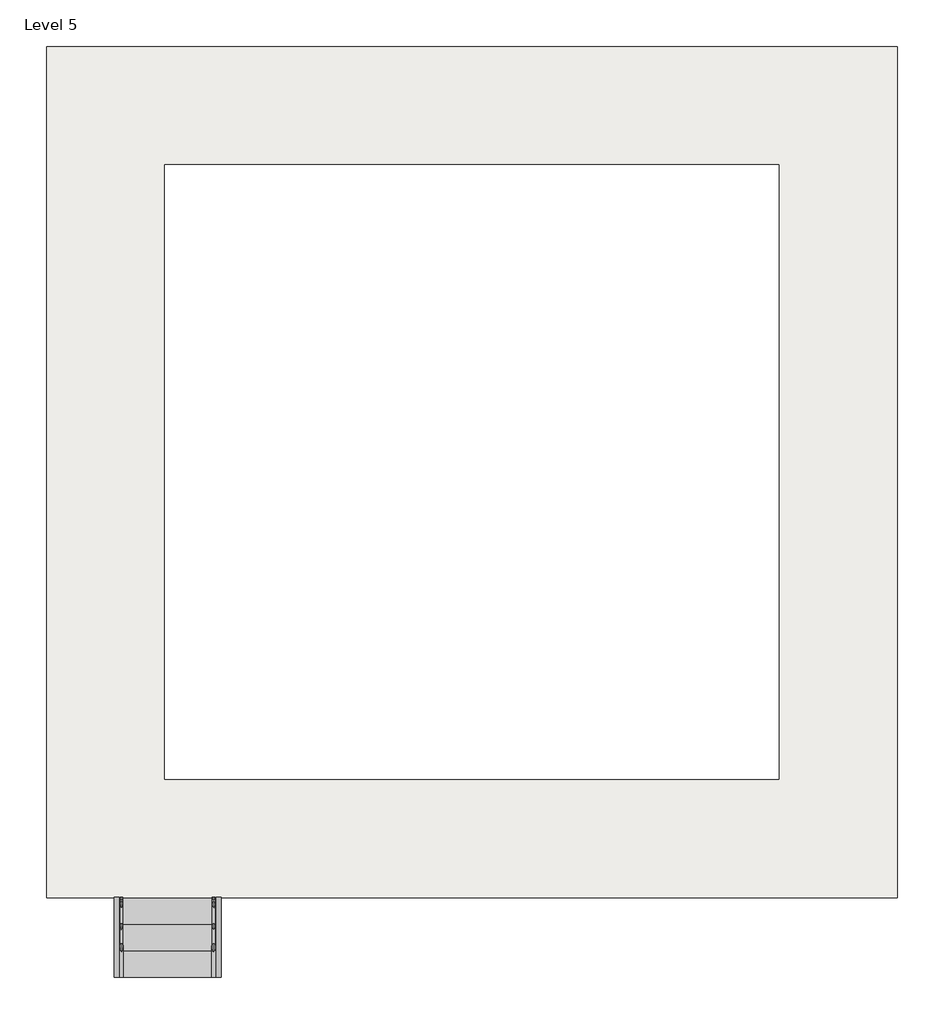
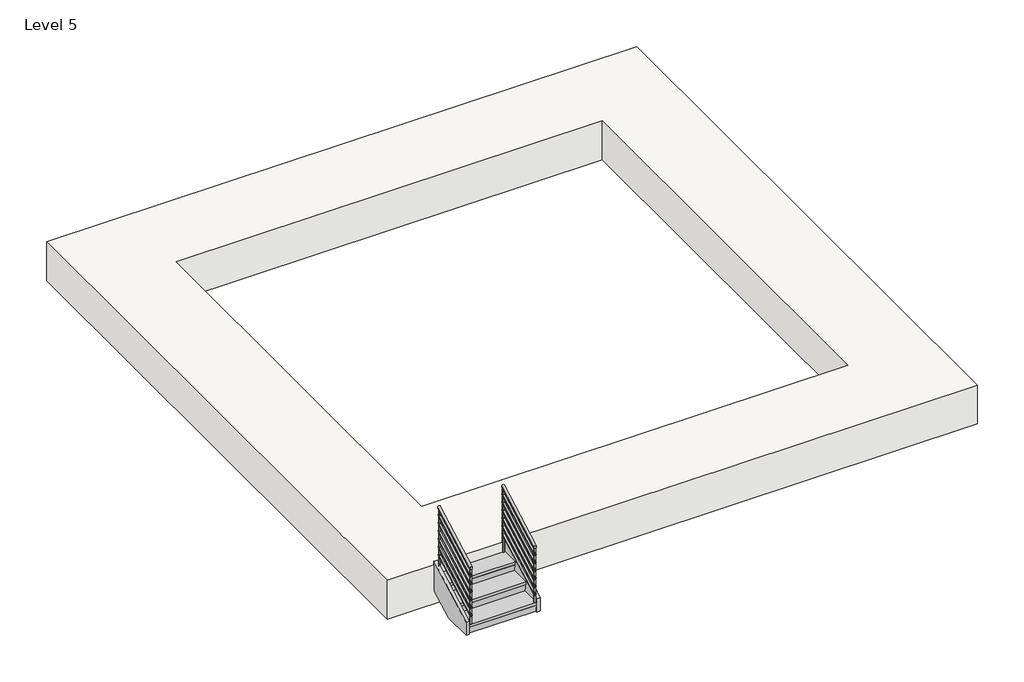
# One storey: 2 members, 2 railings, 1 slab, 1 stair flight.
"""IFC4 building model written with IfcOpenShell, lengths in millimetres."""

from ifc_helpers import new_model, si_unit, frame, origin, place, context, project, spatial, polyline, circle_curve, ellipse_curve, outline, extrude, transform, mapped, element, save
from ifc_brep_helpers import plane_surface, cylinder_surface, advanced_brep
from components import stair_flight_50mm_tread_25mm_nosing_13mm_riser_f84e0c27

model = new_model("IFC4")

# Units and contexts
model_context = context("Model", 3, world=origin())
ifc_project = project(units=[si_unit("LENGTHUNIT", "METRE", prefix="MILLI")], contexts=[model_context])

# Site, building, storey
site = spatial("IfcSite", under=ifc_project)
building = spatial("IfcBuilding", under=site)
storey = spatial("IfcBuildingStorey", under=building, Name="Level 5", Elevation=-609.6)

# Members
placement = place(None, origin())
element("IfcMember", 1, ObjectType="Stringer - 50mm Width", at=placement, inside=storey, context=model_context, shape_type="SweptSolid", body=[
    extrude(outline(polyline([(-5656.14356, -609.6), (-5656.14356, -401.4833471), (-4831.14356, 55.7166529), (-4831.14356, -401.6003029), (-5206.4710976, -609.6), (-5656.14356, -609.6)])), frame((-15823.6523905, 0.0, 0.0), z_axis=(1.0, 0.0, 0.0), x_axis=(0.0, 1.0, 0.0)), (0.0, 0.0, 1.0), 50.0),
])
element("IfcMember", 2, ObjectType="Stringer - 50mm Width", at=placement, inside=storey, context=model_context, shape_type="SweptSolid", body=[
    extrude(outline(polyline([(-5656.14356, -609.6), (-5656.14356, -401.4833471), (-4831.14356, 55.7166529), (-4831.14356, -401.6003029), (-5206.4710976, -609.6), (-5656.14356, -609.6)])), frame((-14773.6266093, 0.0, 0.0), z_axis=(1.0, 0.0, 0.0), x_axis=(0.0, 1.0, 0.0)), (0.0, 0.0, 1.0), 50.0),
])

# Railings
element("IfcRailing", 3, ObjectType="900mm Pipe", at=placement, inside=storey, context=model_context, shape_type="AdvancedBrep", body=[
    advanced_brep(
    [(-14779.0266093, -5656.14356, 419.9341522), (-14819.0266093, -5656.14356, 419.9341522), (-14779.0266093, -4831.14356, 877.1341522), (-14819.0266093, -4831.14356, 877.1341522)],
    [
        (0, 1, ellipse_curve(frame((-14799.0266093, -5656.14356, 419.9341522), z_axis=(0.0, -1.0, 0.0), x_axis=(0.0, 0.0, -0.9999999999999999)), 22.8658478, 20.0)),
        (1, 0, ellipse_curve(frame((-14799.0266093, -5656.14356, 419.9341522), z_axis=(0.0, -1.0, 0.0), x_axis=(0.0, 0.0, -0.9999999999999999)), 22.8658478, 20.0)),
        (2, 3, ellipse_curve(frame((-14799.0266093, -4831.14356, 877.1341522), z_axis=(0.0, 1.0, 0.0), x_axis=(0.0, 0.0, -0.9999999999999999)), 22.8658478, 20.0)),
        (3, 2, ellipse_curve(frame((-14799.0266093, -4831.14356, 877.1341522), z_axis=(0.0, 1.0, 0.0), x_axis=(0.0, 0.0, -0.9999999999999999)), 22.8658478, 20.0)),
        (0, 2),
        (3, 1),
    ],
    [
        plane_surface(frame((-14799.0266093, -5656.14356, 442.8), z_axis=(0.0, -1.0, 0.0), x_axis=(0.0, 0.0, 1.0))),
        plane_surface(frame((-14799.0266093, -4831.14356, 900.0), z_axis=(0.0, 1.0, 0.0), x_axis=(0.0, 0.0, 1.0))),
        cylinder_surface(frame((-14799.0266093, -5646.4490703, 425.3066622), z_axis=(0.0, -0.8746668912460589, -0.48472448809396357), x_axis=(-1.0, 0.0, 0.0)), 20.0),
    ],
    [
        (0, [[1, 2]]),
        (1, [[3, 4]]),
        (2, [[-1, 5, -4, 6]]),
        (2, [[-2, -6, -3, -5]]),
    ],
),
    advanced_brep(
    [(-14814.0266093, -5656.14356, 300.6506142), (-14784.0266093, -5656.14356, 300.6506142), (-14814.0266093, -4831.14356, 757.8506142), (-14784.0266093, -4831.14356, 757.8506142)],
    [
        (0, 1, ellipse_curve(frame((-14799.0266093, -5656.14356, 300.6506142), z_axis=(0.0, -1.0, 0.0), x_axis=(0.0, 0.0, -0.9999999999999999)), 17.1493858, 15.0)),
        (1, 0, ellipse_curve(frame((-14799.0266093, -5656.14356, 300.6506142), z_axis=(0.0, -1.0, 0.0), x_axis=(0.0, 0.0, -0.9999999999999999)), 17.1493858, 15.0)),
        (2, 3, ellipse_curve(frame((-14799.0266093, -4831.14356, 757.8506142), z_axis=(0.0, 1.0, 0.0), x_axis=(0.0, 0.0, -0.9999999999999999)), 17.1493858, 15.0)),
        (3, 2, ellipse_curve(frame((-14799.0266093, -4831.14356, 757.8506142), z_axis=(0.0, 1.0, 0.0), x_axis=(0.0, 0.0, -0.9999999999999999)), 17.1493858, 15.0)),
        (0, 2),
        (3, 1),
    ],
    [
        plane_surface(frame((-14799.0266093, -5656.14356, 317.8), z_axis=(0.0, -1.0, 0.0), x_axis=(0.0, 0.0, 1.0))),
        plane_surface(frame((-14799.0266093, -4831.14356, 775.0), z_axis=(0.0, 1.0, 0.0), x_axis=(0.0, 0.0, 1.0))),
        cylinder_surface(frame((-14799.0266093, -5648.8726927, 304.6799966), z_axis=(0.0, -0.8746668912460589, -0.48472448809396357), x_axis=(1.0, 0.0, 0.0)), 15.0),
    ],
    [
        (0, [[1, 2]]),
        (1, [[3, 4]]),
        (2, [[-1, 5, -4, 6]]),
        (2, [[-2, -6, -3, -5]]),
    ],
),
    advanced_brep(
    [(-14814.0266093, -5656.14356, 175.6506142), (-14784.0266093, -5656.14356, 175.6506142), (-14814.0266093, -4831.14356, 632.8506142), (-14784.0266093, -4831.14356, 632.8506142)],
    [
        (0, 1, ellipse_curve(frame((-14799.0266093, -5656.14356, 175.6506142), z_axis=(0.0, -1.0, 0.0), x_axis=(0.0, 0.0, -0.9999999999999999)), 17.1493858, 15.0)),
        (1, 0, ellipse_curve(frame((-14799.0266093, -5656.14356, 175.6506142), z_axis=(0.0, -1.0, 0.0), x_axis=(0.0, 0.0, -0.9999999999999999)), 17.1493858, 15.0)),
        (2, 3, ellipse_curve(frame((-14799.0266093, -4831.14356, 632.8506142), z_axis=(0.0, 1.0, 0.0), x_axis=(0.0, 0.0, -0.9999999999999999)), 17.1493858, 15.0)),
        (3, 2, ellipse_curve(frame((-14799.0266093, -4831.14356, 632.8506142), z_axis=(0.0, 1.0, 0.0), x_axis=(0.0, 0.0, -0.9999999999999999)), 17.1493858, 15.0)),
        (0, 2),
        (3, 1),
    ],
    [
        plane_surface(frame((-14799.0266093, -5656.14356, 192.8), z_axis=(0.0, -1.0, 0.0), x_axis=(0.0, 0.0, 1.0))),
        plane_surface(frame((-14799.0266093, -4831.14356, 650.0), z_axis=(0.0, 1.0, 0.0), x_axis=(0.0, 0.0, 1.0))),
        cylinder_surface(frame((-14799.0266093, -5648.8726927, 179.6799966), z_axis=(0.0, -0.8746668912460589, -0.48472448809396357), x_axis=(1.0, 0.0, 0.0)), 15.0),
    ],
    [
        (0, [[1, 2]]),
        (1, [[3, 4]]),
        (2, [[-1, 5, -4, 6]]),
        (2, [[-2, -6, -3, -5]]),
    ],
),
    advanced_brep(
    [(-14814.0266093, -5656.14356, 50.6506142), (-14784.0266093, -5656.14356, 50.6506142), (-14814.0266093, -4831.14356, 507.8506142), (-14784.0266093, -4831.14356, 507.8506142)],
    [
        (0, 1, ellipse_curve(frame((-14799.0266093, -5656.14356, 50.6506142), z_axis=(0.0, -1.0, 0.0), x_axis=(0.0, 0.0, -0.9999999999999999)), 17.1493858, 15.0)),
        (1, 0, ellipse_curve(frame((-14799.0266093, -5656.14356, 50.6506142), z_axis=(0.0, -1.0, 0.0), x_axis=(0.0, 0.0, -0.9999999999999999)), 17.1493858, 15.0)),
        (2, 3, ellipse_curve(frame((-14799.0266093, -4831.14356, 507.8506142), z_axis=(0.0, 1.0, 0.0), x_axis=(0.0, 0.0, -0.9999999999999999)), 17.1493858, 15.0)),
        (3, 2, ellipse_curve(frame((-14799.0266093, -4831.14356, 507.8506142), z_axis=(0.0, 1.0, 0.0), x_axis=(0.0, 0.0, -0.9999999999999999)), 17.1493858, 15.0)),
        (0, 2),
        (3, 1),
    ],
    [
        plane_surface(frame((-14799.0266093, -5656.14356, 67.8), z_axis=(0.0, -1.0, 0.0), x_axis=(0.0, 0.0, 1.0))),
        plane_surface(frame((-14799.0266093, -4831.14356, 525.0), z_axis=(0.0, 1.0, 0.0), x_axis=(0.0, 0.0, 1.0))),
        cylinder_surface(frame((-14799.0266093, -5648.8726927, 54.6799966), z_axis=(0.0, -0.8746668912460589, -0.48472448809396357), x_axis=(1.0, 0.0, 0.0)), 15.0),
    ],
    [
        (0, [[1, 2]]),
        (1, [[3, 4]]),
        (2, [[-1, 5, -4, 6]]),
        (2, [[-2, -6, -3, -5]]),
    ],
),
    advanced_brep(
    [(-14814.0266093, -5656.14356, -74.3493858), (-14784.0266093, -5656.14356, -74.3493858), (-14814.0266093, -4831.14356, 382.8506142), (-14784.0266093, -4831.14356, 382.8506142)],
    [
        (0, 1, ellipse_curve(frame((-14799.0266093, -5656.14356, -74.3493858), z_axis=(0.0, -1.0, 0.0), x_axis=(0.0, 0.0, -0.9999999999999999)), 17.1493858, 15.0)),
        (1, 0, ellipse_curve(frame((-14799.0266093, -5656.14356, -74.3493858), z_axis=(0.0, -1.0, 0.0), x_axis=(0.0, 0.0, -0.9999999999999999)), 17.1493858, 15.0)),
        (2, 3, ellipse_curve(frame((-14799.0266093, -4831.14356, 382.8506142), z_axis=(0.0, 1.0, 0.0), x_axis=(0.0, 0.0, -0.9999999999999999)), 17.1493858, 15.0)),
        (3, 2, ellipse_curve(frame((-14799.0266093, -4831.14356, 382.8506142), z_axis=(0.0, 1.0, 0.0), x_axis=(0.0, 0.0, -0.9999999999999999)), 17.1493858, 15.0)),
        (0, 2),
        (3, 1),
    ],
    [
        plane_surface(frame((-14799.0266093, -5656.14356, -57.2), z_axis=(0.0, -1.0, 0.0), x_axis=(0.0, 0.0, 1.0))),
        plane_surface(frame((-14799.0266093, -4831.14356, 400.0), z_axis=(0.0, 1.0, 0.0), x_axis=(0.0, 0.0, 1.0))),
        cylinder_surface(frame((-14799.0266093, -5648.8726927, -70.3200034), z_axis=(0.0, -0.8746668912460589, -0.48472448809396357), x_axis=(1.0, 0.0, 0.0)), 15.0),
    ],
    [
        (0, [[1, 2]]),
        (1, [[3, 4]]),
        (2, [[-1, 5, -4, 6]]),
        (2, [[-2, -6, -3, -5]]),
    ],
),
    advanced_brep(
    [(-14814.0266093, -5656.14356, -199.3493858), (-14784.0266093, -5656.14356, -199.3493858), (-14814.0266093, -4831.14356, 257.8506142), (-14784.0266093, -4831.14356, 257.8506142)],
    [
        (0, 1, ellipse_curve(frame((-14799.0266093, -5656.14356, -199.3493858), z_axis=(0.0, -1.0, 0.0), x_axis=(0.0, 0.0, -0.9999999999999999)), 17.1493858, 15.0)),
        (1, 0, ellipse_curve(frame((-14799.0266093, -5656.14356, -199.3493858), z_axis=(0.0, -1.0, 0.0), x_axis=(0.0, 0.0, -0.9999999999999999)), 17.1493858, 15.0)),
        (2, 3, ellipse_curve(frame((-14799.0266093, -4831.14356, 257.8506142), z_axis=(0.0, 1.0, 0.0), x_axis=(0.0, 0.0, -0.9999999999999999)), 17.1493858, 15.0)),
        (3, 2, ellipse_curve(frame((-14799.0266093, -4831.14356, 257.8506142), z_axis=(0.0, 1.0, 0.0), x_axis=(0.0, 0.0, -0.9999999999999999)), 17.1493858, 15.0)),
        (0, 2),
        (3, 1),
    ],
    [
        plane_surface(frame((-14799.0266093, -5656.14356, -182.2), z_axis=(0.0, -1.0, 0.0), x_axis=(0.0, 0.0, 1.0))),
        plane_surface(frame((-14799.0266093, -4831.14356, 275.0), z_axis=(0.0, 1.0, 0.0), x_axis=(0.0, 0.0, 1.0))),
        cylinder_surface(frame((-14799.0266093, -5648.8726927, -195.3200034), z_axis=(0.0, -0.8746668912460589, -0.48472448809396357), x_axis=(1.0, 0.0, 0.0)), 15.0),
    ],
    [
        (0, [[1, 2]]),
        (1, [[3, 4]]),
        (2, [[-1, 5, -4, 6]]),
        (2, [[-2, -6, -3, -5]]),
    ],
),
    advanced_brep(
    [(-14814.0266093, -5656.14356, -324.3493858), (-14784.0266093, -5656.14356, -324.3493858), (-14814.0266093, -4831.14356, 132.8506142), (-14784.0266093, -4831.14356, 132.8506142)],
    [
        (0, 1, ellipse_curve(frame((-14799.0266093, -5656.14356, -324.3493858), z_axis=(0.0, -1.0, 0.0), x_axis=(0.0, 0.0, -0.9999999999999999)), 17.1493858, 15.0)),
        (1, 0, ellipse_curve(frame((-14799.0266093, -5656.14356, -324.3493858), z_axis=(0.0, -1.0, 0.0), x_axis=(0.0, 0.0, -0.9999999999999999)), 17.1493858, 15.0)),
        (2, 3, ellipse_curve(frame((-14799.0266093, -4831.14356, 132.8506142), z_axis=(0.0, 1.0, 0.0), x_axis=(0.0, 0.0, -0.9999999999999999)), 17.1493858, 15.0)),
        (3, 2, ellipse_curve(frame((-14799.0266093, -4831.14356, 132.8506142), z_axis=(0.0, 1.0, 0.0), x_axis=(0.0, 0.0, -0.9999999999999999)), 17.1493858, 15.0)),
        (0, 2),
        (3, 1),
    ],
    [
        plane_surface(frame((-14799.0266093, -5656.14356, -307.2), z_axis=(0.0, -1.0, 0.0), x_axis=(0.0, 0.0, 1.0))),
        plane_surface(frame((-14799.0266093, -4831.14356, 150.0), z_axis=(0.0, 1.0, 0.0), x_axis=(0.0, 0.0, 1.0))),
        cylinder_surface(frame((-14799.0266093, -5648.8726927, -320.3200034), z_axis=(0.0, -0.8746668912460589, -0.48472448809396357), x_axis=(1.0, 0.0, 0.0)), 15.0),
    ],
    [
        (0, [[1, 2]]),
        (1, [[3, 4]]),
        (2, [[-1, 5, -4, 6]]),
        (2, [[-2, -6, -3, -5]]),
    ],
),
    advanced_brep(
    [(-14786.5266093, -4843.64356, 847.3410317), (-14786.5266093, -4843.64356, -152.4), (-14811.5266093, -4843.64356, -152.4), (-14811.5266093, -4843.64356, 847.3410317)],
    [
        (0, 1),
        (1, 2, circle_curve(frame((-14799.0266093, -4843.64356, -152.4), z_axis=(0.0, 0.0, 1.0), x_axis=(-1.0, 0.0, 0.0)), 12.5)),
        (2, 3),
        (3, 0, ellipse_curve(frame((-14799.0266093, -4843.64356, 847.3410317), z_axis=(0.0, 0.48472448809396185, -0.8746668912460599), x_axis=(0.0, 0.8746668912460599, 0.48472448809396146)), 14.2911549, 12.5)),
        (0, 3, ellipse_curve(frame((-14799.0266093, -4843.64356, 847.3410317), z_axis=(0.0, 0.48472448809396185, -0.8746668912460599), x_axis=(0.0, 0.8746668912460599, 0.48472448809396146)), 14.2911549, 12.5)),
        (2, 1, circle_curve(frame((-14799.0266093, -4843.64356, -152.4), z_axis=(0.0, 0.0, 1.0), x_axis=(-1.0, 0.0, 0.0)), 12.5)),
    ],
    [
        cylinder_surface(frame((-14799.0266093, -4843.64356, -252.4), z_axis=(0.0, 0.0, 1.0), x_axis=(-1.0, 0.0, 0.0)), 12.5),
        plane_surface(frame((-14824.0266093, -4818.64356, 861.1955772), z_axis=(0.0, -0.48472448809396185, 0.8746668912460599), x_axis=(1.0, 0.0, 0.0))),
        plane_surface(frame((-14824.0266093, -4868.64356, -152.4), z_axis=(0.0, 0.0, -1.0), x_axis=(1.0, 0.0, 0.0))),
    ],
    [
        (0, [[1, 2, 3, 4]]),
        (0, [[-1, 5, -3, 6]]),
        (1, [[-4, -5]]),
        (2, [[-2, -6]]),
    ],
),
    advanced_brep(
    [(-14786.5266093, -5643.64356, 403.9955772), (-14786.5266093, -5643.64356, -457.2), (-14811.5266093, -5643.64356, -457.2), (-14811.5266093, -5643.64356, 403.9955772)],
    [
        (0, 1),
        (1, 2, circle_curve(frame((-14799.0266093, -5643.64356, -457.2), z_axis=(0.0, 0.0, 1.0), x_axis=(-1.0, 0.0, 0.0)), 12.5)),
        (2, 3),
        (3, 0, ellipse_curve(frame((-14799.0266093, -5643.64356, 403.9955772), z_axis=(0.0, 0.48472448809396185, -0.8746668912460599), x_axis=(0.0, 0.8746668912460599, 0.48472448809396146)), 14.2911549, 12.5)),
        (0, 3, ellipse_curve(frame((-14799.0266093, -5643.64356, 403.9955772), z_axis=(0.0, 0.48472448809396185, -0.8746668912460599), x_axis=(0.0, 0.8746668912460599, 0.48472448809396146)), 14.2911549, 12.5)),
        (2, 1, circle_curve(frame((-14799.0266093, -5643.64356, -457.2), z_axis=(0.0, 0.0, 1.0), x_axis=(-1.0, 0.0, 0.0)), 12.5)),
    ],
    [
        cylinder_surface(frame((-14799.0266093, -5643.64356, -557.2), z_axis=(0.0, 0.0, 1.0), x_axis=(-1.0, 0.0, 0.0)), 12.5),
        plane_surface(frame((-14824.0266093, -5618.64356, 417.8501226), z_axis=(0.0, -0.48472448809396185, 0.8746668912460599), x_axis=(1.0, 0.0, 0.0))),
        plane_surface(frame((-14824.0266093, -5668.64356, -457.2), z_axis=(0.0, 0.0, -1.0), x_axis=(1.0, 0.0, 0.0))),
    ],
    [
        (0, [[1, 2, 3, 4]]),
        (0, [[-1, 5, -3, 6]]),
        (1, [[-4, -5]]),
        (2, [[-2, -6]]),
    ],
),
])
element("IfcRailing", 4, ObjectType="900mm Pipe", at=placement, inside=storey, context=model_context, shape_type="AdvancedBrep", body=[
    advanced_brep(
    [(-15728.2523905, -5656.14356, 419.9341522), (-15768.2523905, -5656.14356, 419.9341522), (-15728.2523905, -4831.14356, 877.1341522), (-15768.2523905, -4831.14356, 877.1341522)],
    [
        (0, 1, ellipse_curve(frame((-15748.2523905, -5656.14356, 419.9341522), z_axis=(0.0, -1.0, 0.0), x_axis=(0.0, 0.0, -0.9999999999999999)), 22.8658478, 20.0)),
        (1, 0, ellipse_curve(frame((-15748.2523905, -5656.14356, 419.9341522), z_axis=(0.0, -1.0, 0.0), x_axis=(0.0, 0.0, -0.9999999999999999)), 22.8658478, 20.0)),
        (2, 3, ellipse_curve(frame((-15748.2523905, -4831.14356, 877.1341522), z_axis=(0.0, 1.0, 0.0), x_axis=(0.0, 0.0, -0.9999999999999999)), 22.8658478, 20.0)),
        (3, 2, ellipse_curve(frame((-15748.2523905, -4831.14356, 877.1341522), z_axis=(0.0, 1.0, 0.0), x_axis=(0.0, 0.0, -0.9999999999999999)), 22.8658478, 20.0)),
        (0, 2),
        (3, 1),
    ],
    [
        plane_surface(frame((-15748.2523905, -5656.14356, 442.8), z_axis=(0.0, -1.0, 0.0), x_axis=(0.0, 0.0, 1.0))),
        plane_surface(frame((-15748.2523905, -4831.14356, 900.0), z_axis=(0.0, 1.0, 0.0), x_axis=(0.0, 0.0, 1.0))),
        cylinder_surface(frame((-15748.2523905, -5646.4490703, 425.3066622), z_axis=(0.0, -0.8746668912460589, -0.48472448809396357), x_axis=(-1.0, 0.0, 0.0)), 20.0),
    ],
    [
        (0, [[1, 2]]),
        (1, [[3, 4]]),
        (2, [[-1, 5, -4, 6]]),
        (2, [[-2, -6, -3, -5]]),
    ],
),
    advanced_brep(
    [(-15733.2523905, -5656.14356, 300.6506142), (-15763.2523905, -5656.14356, 300.6506142), (-15733.2523905, -4831.14356, 757.8506142), (-15763.2523905, -4831.14356, 757.8506142)],
    [
        (0, 1, ellipse_curve(frame((-15748.2523905, -5656.14356, 300.6506142), z_axis=(0.0, -1.0, 0.0), x_axis=(0.0, 0.0, -0.9999999999999999)), 17.1493858, 15.0)),
        (1, 0, ellipse_curve(frame((-15748.2523905, -5656.14356, 300.6506142), z_axis=(0.0, -1.0, 0.0), x_axis=(0.0, 0.0, -0.9999999999999999)), 17.1493858, 15.0)),
        (2, 3, ellipse_curve(frame((-15748.2523905, -4831.14356, 757.8506142), z_axis=(0.0, 1.0, 0.0), x_axis=(0.0, 0.0, -0.9999999999999999)), 17.1493858, 15.0)),
        (3, 2, ellipse_curve(frame((-15748.2523905, -4831.14356, 757.8506142), z_axis=(0.0, 1.0, 0.0), x_axis=(0.0, 0.0, -0.9999999999999999)), 17.1493858, 15.0)),
        (0, 2),
        (3, 1),
    ],
    [
        plane_surface(frame((-15748.2523905, -5656.14356, 317.8), z_axis=(0.0, -1.0, 0.0), x_axis=(0.0, 0.0, 1.0))),
        plane_surface(frame((-15748.2523905, -4831.14356, 775.0), z_axis=(0.0, 1.0, 0.0), x_axis=(0.0, 0.0, 1.0))),
        cylinder_surface(frame((-15748.2523905, -5648.8726927, 304.6799966), z_axis=(0.0, -0.8746668912460589, -0.48472448809396357), x_axis=(-1.0, 0.0, 0.0)), 15.0),
    ],
    [
        (0, [[1, 2]]),
        (1, [[3, 4]]),
        (2, [[-1, 5, -4, 6]]),
        (2, [[-2, -6, -3, -5]]),
    ],
),
    advanced_brep(
    [(-15733.2523905, -5656.14356, 175.6506142), (-15763.2523905, -5656.14356, 175.6506142), (-15733.2523905, -4831.14356, 632.8506142), (-15763.2523905, -4831.14356, 632.8506142)],
    [
        (0, 1, ellipse_curve(frame((-15748.2523905, -5656.14356, 175.6506142), z_axis=(0.0, -1.0, 0.0), x_axis=(0.0, 0.0, -0.9999999999999999)), 17.1493858, 15.0)),
        (1, 0, ellipse_curve(frame((-15748.2523905, -5656.14356, 175.6506142), z_axis=(0.0, -1.0, 0.0), x_axis=(0.0, 0.0, -0.9999999999999999)), 17.1493858, 15.0)),
        (2, 3, ellipse_curve(frame((-15748.2523905, -4831.14356, 632.8506142), z_axis=(0.0, 1.0, 0.0), x_axis=(0.0, 0.0, -0.9999999999999999)), 17.1493858, 15.0)),
        (3, 2, ellipse_curve(frame((-15748.2523905, -4831.14356, 632.8506142), z_axis=(0.0, 1.0, 0.0), x_axis=(0.0, 0.0, -0.9999999999999999)), 17.1493858, 15.0)),
        (0, 2),
        (3, 1),
    ],
    [
        plane_surface(frame((-15748.2523905, -5656.14356, 192.8), z_axis=(0.0, -1.0, 0.0), x_axis=(0.0, 0.0, 1.0))),
        plane_surface(frame((-15748.2523905, -4831.14356, 650.0), z_axis=(0.0, 1.0, 0.0), x_axis=(0.0, 0.0, 1.0))),
        cylinder_surface(frame((-15748.2523905, -5648.8726927, 179.6799966), z_axis=(0.0, -0.8746668912460589, -0.48472448809396357), x_axis=(-1.0, 0.0, 0.0)), 15.0),
    ],
    [
        (0, [[1, 2]]),
        (1, [[3, 4]]),
        (2, [[-1, 5, -4, 6]]),
        (2, [[-2, -6, -3, -5]]),
    ],
),
    advanced_brep(
    [(-15733.2523905, -5656.14356, 50.6506142), (-15763.2523905, -5656.14356, 50.6506142), (-15733.2523905, -4831.14356, 507.8506142), (-15763.2523905, -4831.14356, 507.8506142)],
    [
        (0, 1, ellipse_curve(frame((-15748.2523905, -5656.14356, 50.6506142), z_axis=(0.0, -1.0, 0.0), x_axis=(0.0, 0.0, -0.9999999999999999)), 17.1493858, 15.0)),
        (1, 0, ellipse_curve(frame((-15748.2523905, -5656.14356, 50.6506142), z_axis=(0.0, -1.0, 0.0), x_axis=(0.0, 0.0, -0.9999999999999999)), 17.1493858, 15.0)),
        (2, 3, ellipse_curve(frame((-15748.2523905, -4831.14356, 507.8506142), z_axis=(0.0, 1.0, 0.0), x_axis=(0.0, 0.0, -0.9999999999999999)), 17.1493858, 15.0)),
        (3, 2, ellipse_curve(frame((-15748.2523905, -4831.14356, 507.8506142), z_axis=(0.0, 1.0, 0.0), x_axis=(0.0, 0.0, -0.9999999999999999)), 17.1493858, 15.0)),
        (0, 2),
        (3, 1),
    ],
    [
        plane_surface(frame((-15748.2523905, -5656.14356, 67.8), z_axis=(0.0, -1.0, 0.0), x_axis=(0.0, 0.0, 1.0))),
        plane_surface(frame((-15748.2523905, -4831.14356, 525.0), z_axis=(0.0, 1.0, 0.0), x_axis=(0.0, 0.0, 1.0))),
        cylinder_surface(frame((-15748.2523905, -5648.8726927, 54.6799966), z_axis=(0.0, -0.8746668912460589, -0.48472448809396357), x_axis=(-1.0, 0.0, 0.0)), 15.0),
    ],
    [
        (0, [[1, 2]]),
        (1, [[3, 4]]),
        (2, [[-1, 5, -4, 6]]),
        (2, [[-2, -6, -3, -5]]),
    ],
),
    advanced_brep(
    [(-15733.2523905, -5656.14356, -74.3493858), (-15763.2523905, -5656.14356, -74.3493858), (-15733.2523905, -4831.14356, 382.8506142), (-15763.2523905, -4831.14356, 382.8506142)],
    [
        (0, 1, ellipse_curve(frame((-15748.2523905, -5656.14356, -74.3493858), z_axis=(0.0, -1.0, 0.0), x_axis=(0.0, 0.0, -0.9999999999999999)), 17.1493858, 15.0)),
        (1, 0, ellipse_curve(frame((-15748.2523905, -5656.14356, -74.3493858), z_axis=(0.0, -1.0, 0.0), x_axis=(0.0, 0.0, -0.9999999999999999)), 17.1493858, 15.0)),
        (2, 3, ellipse_curve(frame((-15748.2523905, -4831.14356, 382.8506142), z_axis=(0.0, 1.0, 0.0), x_axis=(0.0, 0.0, -0.9999999999999999)), 17.1493858, 15.0)),
        (3, 2, ellipse_curve(frame((-15748.2523905, -4831.14356, 382.8506142), z_axis=(0.0, 1.0, 0.0), x_axis=(0.0, 0.0, -0.9999999999999999)), 17.1493858, 15.0)),
        (0, 2),
        (3, 1),
    ],
    [
        plane_surface(frame((-15748.2523905, -5656.14356, -57.2), z_axis=(0.0, -1.0, 0.0), x_axis=(0.0, 0.0, 1.0))),
        plane_surface(frame((-15748.2523905, -4831.14356, 400.0), z_axis=(0.0, 1.0, 0.0), x_axis=(0.0, 0.0, 1.0))),
        cylinder_surface(frame((-15748.2523905, -5648.8726927, -70.3200034), z_axis=(0.0, -0.8746668912460589, -0.48472448809396357), x_axis=(-1.0, 0.0, 0.0)), 15.0),
    ],
    [
        (0, [[1, 2]]),
        (1, [[3, 4]]),
        (2, [[-1, 5, -4, 6]]),
        (2, [[-2, -6, -3, -5]]),
    ],
),
    advanced_brep(
    [(-15733.2523905, -5656.14356, -199.3493858), (-15763.2523905, -5656.14356, -199.3493858), (-15733.2523905, -4831.14356, 257.8506142), (-15763.2523905, -4831.14356, 257.8506142)],
    [
        (0, 1, ellipse_curve(frame((-15748.2523905, -5656.14356, -199.3493858), z_axis=(0.0, -1.0, 0.0), x_axis=(0.0, 0.0, -0.9999999999999999)), 17.1493858, 15.0)),
        (1, 0, ellipse_curve(frame((-15748.2523905, -5656.14356, -199.3493858), z_axis=(0.0, -1.0, 0.0), x_axis=(0.0, 0.0, -0.9999999999999999)), 17.1493858, 15.0)),
        (2, 3, ellipse_curve(frame((-15748.2523905, -4831.14356, 257.8506142), z_axis=(0.0, 1.0, 0.0), x_axis=(0.0, 0.0, -0.9999999999999999)), 17.1493858, 15.0)),
        (3, 2, ellipse_curve(frame((-15748.2523905, -4831.14356, 257.8506142), z_axis=(0.0, 1.0, 0.0), x_axis=(0.0, 0.0, -0.9999999999999999)), 17.1493858, 15.0)),
        (0, 2),
        (3, 1),
    ],
    [
        plane_surface(frame((-15748.2523905, -5656.14356, -182.2), z_axis=(0.0, -1.0, 0.0), x_axis=(0.0, 0.0, 1.0))),
        plane_surface(frame((-15748.2523905, -4831.14356, 275.0), z_axis=(0.0, 1.0, 0.0), x_axis=(0.0, 0.0, 1.0))),
        cylinder_surface(frame((-15748.2523905, -5648.8726927, -195.3200034), z_axis=(0.0, -0.8746668912460589, -0.48472448809396357), x_axis=(-1.0, 0.0, 0.0)), 15.0),
    ],
    [
        (0, [[1, 2]]),
        (1, [[3, 4]]),
        (2, [[-1, 5, -4, 6]]),
        (2, [[-2, -6, -3, -5]]),
    ],
),
    advanced_brep(
    [(-15733.2523905, -5656.14356, -324.3493858), (-15763.2523905, -5656.14356, -324.3493858), (-15733.2523905, -4831.14356, 132.8506142), (-15763.2523905, -4831.14356, 132.8506142)],
    [
        (0, 1, ellipse_curve(frame((-15748.2523905, -5656.14356, -324.3493858), z_axis=(0.0, -1.0, 0.0), x_axis=(0.0, 0.0, -0.9999999999999999)), 17.1493858, 15.0)),
        (1, 0, ellipse_curve(frame((-15748.2523905, -5656.14356, -324.3493858), z_axis=(0.0, -1.0, 0.0), x_axis=(0.0, 0.0, -0.9999999999999999)), 17.1493858, 15.0)),
        (2, 3, ellipse_curve(frame((-15748.2523905, -4831.14356, 132.8506142), z_axis=(0.0, 1.0, 0.0), x_axis=(0.0, 0.0, -0.9999999999999999)), 17.1493858, 15.0)),
        (3, 2, ellipse_curve(frame((-15748.2523905, -4831.14356, 132.8506142), z_axis=(0.0, 1.0, 0.0), x_axis=(0.0, 0.0, -0.9999999999999999)), 17.1493858, 15.0)),
        (0, 2),
        (3, 1),
    ],
    [
        plane_surface(frame((-15748.2523905, -5656.14356, -307.2), z_axis=(0.0, -1.0, 0.0), x_axis=(0.0, 0.0, 1.0))),
        plane_surface(frame((-15748.2523905, -4831.14356, 150.0), z_axis=(0.0, 1.0, 0.0), x_axis=(0.0, 0.0, 1.0))),
        cylinder_surface(frame((-15748.2523905, -5648.8726927, -320.3200034), z_axis=(0.0, -0.8746668912460589, -0.48472448809396357), x_axis=(-1.0, 0.0, 0.0)), 15.0),
    ],
    [
        (0, [[1, 2]]),
        (1, [[3, 4]]),
        (2, [[-1, 5, -4, 6]]),
        (2, [[-2, -6, -3, -5]]),
    ],
),
    advanced_brep(
    [(-15760.7523905, -4843.64356, 847.3410317), (-15735.7523905, -4843.64356, 847.3410317), (-15735.7523905, -4843.64356, -152.4), (-15760.7523905, -4843.64356, -152.4)],
    [
        (0, 1, ellipse_curve(frame((-15748.2523905, -4843.64356, 847.3410317), z_axis=(0.0, 0.48472448809396185, -0.8746668912460599), x_axis=(0.0, 0.8746668912460599, 0.48472448809396146)), 14.2911549, 12.5)),
        (1, 2),
        (2, 3, circle_curve(frame((-15748.2523905, -4843.64356, -152.4), z_axis=(0.0, 0.0, 1.0), x_axis=(1.0, 0.0, 0.0)), 12.5)),
        (3, 0),
        (3, 2, circle_curve(frame((-15748.2523905, -4843.64356, -152.4), z_axis=(0.0, 0.0, 1.0), x_axis=(1.0, 0.0, 0.0)), 12.5)),
        (1, 0, ellipse_curve(frame((-15748.2523905, -4843.64356, 847.3410317), z_axis=(0.0, 0.48472448809396185, -0.8746668912460599), x_axis=(0.0, 0.8746668912460599, 0.48472448809396146)), 14.2911549, 12.5)),
    ],
    [
        cylinder_surface(frame((-15748.2523905, -4843.64356, -252.4), z_axis=(0.0, 0.0, 1.0), x_axis=(1.0, 0.0, 0.0)), 12.5),
        plane_surface(frame((-15723.2523905, -4818.64356, 861.1955772), z_axis=(0.0, -0.48472448809396185, 0.8746668912460599), x_axis=(-1.0, 0.0, 0.0))),
        plane_surface(frame((-15723.2523905, -4868.64356, -152.4), z_axis=(0.0, 0.0, -1.0), x_axis=(-1.0, 0.0, 0.0))),
    ],
    [
        (0, [[1, 2, 3, 4]]),
        (0, [[5, -2, 6, -4]]),
        (1, [[-6, -1]]),
        (2, [[-5, -3]]),
    ],
),
    advanced_brep(
    [(-15760.7523905, -5643.64356, 403.9955772), (-15735.7523905, -5643.64356, 403.9955772), (-15735.7523905, -5643.64356, -457.2), (-15760.7523905, -5643.64356, -457.2)],
    [
        (0, 1, ellipse_curve(frame((-15748.2523905, -5643.64356, 403.9955772), z_axis=(0.0, 0.48472448809396185, -0.8746668912460599), x_axis=(0.0, 0.8746668912460599, 0.48472448809396146)), 14.2911549, 12.5)),
        (1, 2),
        (2, 3, circle_curve(frame((-15748.2523905, -5643.64356, -457.2), z_axis=(0.0, 0.0, 1.0), x_axis=(1.0, 0.0, 0.0)), 12.5)),
        (3, 0),
        (3, 2, circle_curve(frame((-15748.2523905, -5643.64356, -457.2), z_axis=(0.0, 0.0, 1.0), x_axis=(1.0, 0.0, 0.0)), 12.5)),
        (1, 0, ellipse_curve(frame((-15748.2523905, -5643.64356, 403.9955772), z_axis=(0.0, 0.48472448809396185, -0.8746668912460599), x_axis=(0.0, 0.8746668912460599, 0.48472448809396146)), 14.2911549, 12.5)),
    ],
    [
        cylinder_surface(frame((-15748.2523905, -5643.64356, -557.2), z_axis=(0.0, 0.0, 1.0), x_axis=(1.0, 0.0, 0.0)), 12.5),
        plane_surface(frame((-15723.2523905, -5618.64356, 417.8501226), z_axis=(0.0, -0.48472448809396185, 0.8746668912460599), x_axis=(-1.0, 0.0, 0.0))),
        plane_surface(frame((-15723.2523905, -5668.64356, -457.2), z_axis=(0.0, 0.0, -1.0), x_axis=(-1.0, 0.0, 0.0))),
    ],
    [
        (0, [[1, 2, 3, 4]]),
        (0, [[5, -2, 6, -4]]),
        (1, [[-6, -1]]),
        (2, [[-5, -3]]),
    ],
),
])

# Slab
element("IfcSlab", 5, ObjectType="PLINTH", at=placement, inside=storey, context=model_context, shape_type="SweptSolid", body=[
    extrude(outline(polyline([(-7756.9443193, -4836.9643531), (-16519.9443193, -4836.9643531), (-16519.9443193, 3926.0356469), (-7756.9443193, 3926.0356469), (-7756.9443193, -4836.9643531)]), holes=[polyline([(-15300.7443193, -3617.7643531), (-8976.1443193, -3617.7643531), (-8976.1443193, 2706.8356469), (-15300.7443193, 2706.8356469), (-15300.7443193, -3617.7643531)])]), frame((0.0, 0.0, -609.6), z_axis=(0.0, 0.0, 1.0), x_axis=(1.0, 0.0, 0.0)), (0.0, 0.0, 1.0), 609.6),
])

# Stair flight
stair_flight_50mm_tread_25mm_nosing_13mm_riser_shape = stair_flight_50mm_tread_25mm_nosing_13mm_riser_f84e0c27(model_context)
element("IfcStairFlight", 6, ObjectType="50mm Tread 25mm Nosing 13mm Riser", at=placement, inside=storey, context=model_context, shape_type="MappedRepresentation", body=[
    mapped(stair_flight_50mm_tread_25mm_nosing_13mm_riser_shape, transform((0.0, 0.0, 0.0), x_axis=(1.0, 0.0, 0.0), y_axis=(0.0, 1.0, 0.0), z_axis=(0.0, 0.0, 1.0))),
])

save(model, "model.ifc")

# Revit data of these elements
# Type "900mm Pipe"
#   built-in parameter 1008612 = 0.019685 (stored number, unit not read)
#   built-in parameter 1008611 = 0.0984252 (stored number, unit not read)
#   built-in parameter 1008609 = 6.56168 (stored number, unit not read)
#   built-in parameter 1008604 = 0.19685 (stored number, unit not read)
#   built-in parameter 1008603 = 0.164042 (stored number, unit not read)
#   Railing Height = 900 mm
#   built-in parameter 1008630 = 2
#   built-in parameter 1008610 = 2
#   built-in parameter 1008605 = 1
#   built-in parameter 1008618 = M_Baluster - Round : 25mm
# Type "PLINTH"
#   Function = 0
#   Layers, outside or top first: 609.6 mm no material (function 1)
# Elements 1, 2 (IfcMember, "Stringer - 50mm Width")
#   Phase Created = New Construction
# Elements 3, 4 (IfcRailing, "900mm Pipe")
#   Phase Created = New Construction
# Element 5 (IfcSlab, "PLINTH")
#   built-in parameter 1001955 = 3.14159 (stored number, unit not read)
#   Height Offset From Level = 609.6 mm
#   Phase Created = New Construction
#   Materials on its faces: "Default Roof"
# Element 6 (IfcStairFlight, "50mm Tread 25mm Nosing 13mm Riser")
#   Phase Created = New Construction
# Materials
#   "Default Roof": colour RGB 80 80 80, transparency 0
